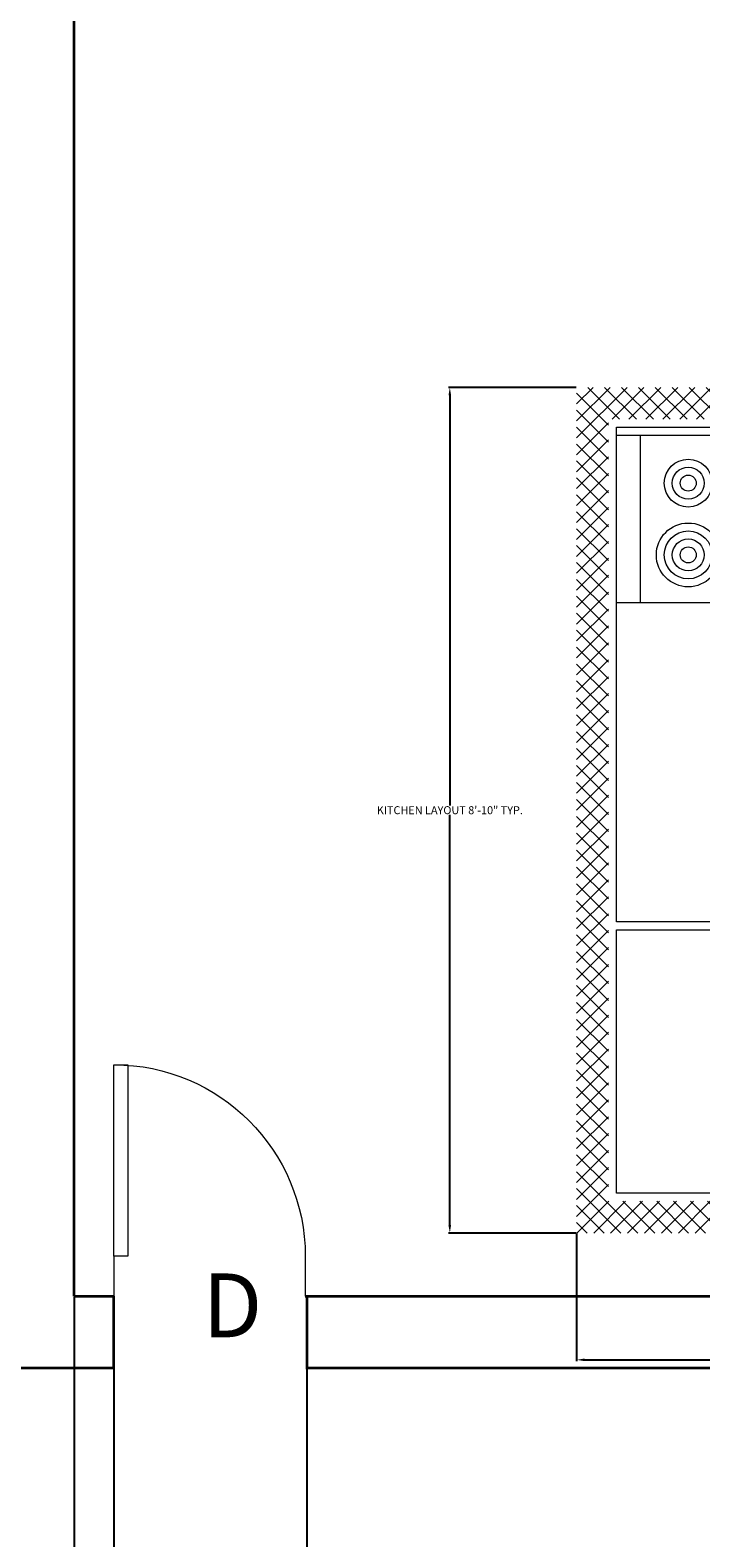
# Model space of a CAD drawing. Units: inches. Extents: x 371 to 1095, y -45 to 1219.
# Tile 11 of 18: x 856 to 940, y 421 to 610. Entities that reach past the tile are written whole.
import ezdxf

# ---------------------------------------------------------------- set-up
doc = ezdxf.new("R2010")
doc.units = ezdxf.units.IN
doc.header["$MEASUREMENT"] = 0
for name, color, linetype, lineweight in [('A-ANNO-DIMS', 2, 'Continuous', 18), ('A-ANNO-TEXT', 7, 'Continuous', 18), ('A-DOOR', 3, 'Continuous', 18), ('A-FLOR-FIXT', 9, 'Continuous', 18), ('A-WALL', 40, 'Continuous', 35)]:
    doc.layers.add(name, color=color, linetype=linetype, lineweight=lineweight)
doc.styles.get("Standard").update_dxf_attribs({"font": 'arial.ttf'})
doc.dimstyles.get("Standard").update_dxf_attribs({"dimtxt": 1, "dimasz": 1, "dimexe": 0.18, "dimexo": 0.0625, "dimgap": 0.09, "dimtad": 0, "dimtih": 1, "dimtoh": 1, "dimdec": 0, "dimzin": 0, "dimdsep": 46, "dimlunit": 3, "dimtxsty": 'Standard', "dimcen": 0.09, "dimadec": 0, "dimazin": 0, "dimtfac": 1, "dimtdec": 0, "dimtofl": 0, "dimtmove": 0, "dimatfit": 3, "dimfxl": 1, "dimtolj": 1, "dimtzin": 0, "dimarcsym": 0})

# ---------------------------------------------------------------- blocks, each defined once
blk = doc.blocks.new('*U12')
for p, q in [((0, 0), (0, 5)), ((24, 0), (24, 5))]:
    blk.add_line(p, q)
blk.add_lwpolyline([(0, 0), (0, -24), (1.75, -24), (1.75, 0)], close=True)
blk.add_arc((0, 0), 24, 270, 0)
blk = doc.blocks.new('Kitchen Layout - 7 x 8 ft')
for p, q in [((-5, 81.32), (2.68, 89)), ((-5, 83.44), (0.56, 89)), ((-5, 85.56), (-1.56, 89)), ((-5, 87.68), (-3.68, 89)), ((-1, 84.97), (-5, 88.97)), ((1.09, 85), (-2.91, 89)), ((3.21, 85), (-0.79, 89)), ((0.81, 85), (4.81, 89)), ((5.34, 85), (1.34, 89)), ((2.93, 85), (6.93, 89)), ((7.46, 85), (3.46, 89)), ((5.05, 85), (9.05, 89)), ((9.58, 85), (5.58, 89)), ((7.17, 85), (11.17, 89)), ((11.7, 85), (7.7, 89)), ((9.29, 85), (13.29, 89)), ((13.82, 85), (9.82, 89)), ((11.41, 85), (15.41, 89)), ((15.94, 85), (11.94, 89)), ((13.53, 85), (17.53, 89)), ((18.06, 85), (14.06, 89)), ((15.65, 85), (19.65, 89)), ((20.18, 85), (16.18, 89)), ((17.78, 85), (21.78, 89)), ((22.31, 85), (18.31, 89)), ((19.9, 85), (23.9, 89)), ((24.43, 85), (20.43, 89)), ((22.02, 85), (26.02, 89)), ((26.55, 85), (22.55, 89)), ((24.14, 85), (28.14, 89)), ((28.67, 85), (24.67, 89)), ((26.26, 85), (30.26, 89)), ((30.79, 85), (26.79, 89)), ((28.38, 85), (32.38, 89)), ((32.91, 85), (28.91, 89)), ((30.5, 85), (34.5, 89)), ((35.03, 85), (31.03, 89)), ((32.63, 85), (36.63, 89)), ((37.16, 85), (33.16, 89)), ((34.75, 85), (38.75, 89)), ((39.28, 85), (35.28, 89)), ((36.87, 85), (40.87, 89)), ((41.4, 85), (37.4, 89)), ((38.99, 85), (42.99, 89)), ((43.52, 85), (39.52, 89)), ((41.11, 85), (45.11, 89)), ((45.64, 85), (41.64, 89)), ((43.23, 85), (47.23, 89)), ((47.76, 85), (43.76, 89)), ((45.35, 85), (49.35, 89)), ((49.88, 85), (45.88, 89)), ((47.47, 85), (51.47, 89)), ((52, 85), (48, 89)), ((49.6, 85), (53.6, 89)), ((54.13, 85), (50.13, 89)), ((51.72, 85), (55.72, 89)), ((56.25, 85), (52.25, 89)), ((53.84, 85), (57.84, 89)), ((58.37, 85), (54.37, 89)), ((55.96, 85), (59.96, 89)), ((60.49, 85), (56.49, 89)), ((58.08, 85), (62.08, 89)), ((62.61, 85), (58.61, 89)), ((60.2, 85), (64.2, 89)), ((64.73, 85), (60.73, 89)), ((62.32, 85), (66.32, 89)), ((66.85, 85), (62.85, 89)), ((64.45, 85), (68.45, 89)), ((68.97, 85), (64.97, 89)), ((66.57, 85), (70.57, 89)), ((71.1, 85), (67.1, 89)), ((68.69, 85), (72.69, 89)), ((73.22, 85), (69.22, 89)), ((70.81, 85), (74.81, 89)), ((75.34, 85), (71.34, 89)), ((72.93, 85), (76.93, 89)), ((77.46, 85), (73.46, 89)), ((75.05, 85), (79.05, 89)), ((79.58, 85), (75.58, 89)), ((77.17, 85), (81.17, 89)), ((81.7, 85), (77.7, 89)), ((79.29, 85), (83.29, 89)), ((83.82, 85), (79.82, 89)), ((81.42, 85), (85.42, 89)), ((85.95, 85), (81.95, 89)), ((83.54, 85), (87.54, 89)), ((88.07, 85), (84.07, 89)), ((85.66, 85), (89.66, 89)), ((90.19, 85), (86.19, 89)), ((87.78, 85), (91.78, 89)), ((92.31, 85), (88.31, 89)), ((89.9, 85), (93.9, 89)), ((94.43, 85), (90.43, 89)), ((92.02, 85), (96.02, 89)), ((96.55, 85), (92.55, 89)), ((94.14, 85), (98.14, 89)), ((101, 82.67), (94.67, 89)), ((96.27, 85), (100.27, 89)), ((101, 84.79), (96.79, 89)), ((101, 86.92), (98.92, 89)), ((97, 83.61), (101, 87.61)), ((-1, 82.85), (-5, 86.85)), ((97, 81.49), (101, 85.49)), ((-1, 80.73), (-5, 84.73)), ((-5, 79.19), (-1, 83.19)), ((34, 84), (96, 84)), ((34, 60), (34, 84)), ((96, 84), (96, 60)), ((101, 80.55), (97, 84.55)), ((97, 79.37), (101, 83.37)), ((-1, 78.61), (-5, 82.61)), ((101, 78.43), (97, 82.43)), ((-5, 77.07), (-1, 81.07)), ((-1, 76.49), (-5, 80.49)), ((74, 81), (95, 81)), ((97, 77.25), (101, 81.25)), ((101, 76.31), (97, 80.31)), ((-5, 74.95), (-1, 78.95)), ((-1, 74.36), (-5, 78.36)), ((97, 75.13), (101, 79.13)), ((101, 74.19), (97, 78.19)), ((-5, 72.83), (-1, 76.83)), ((-1, 72.24), (-5, 76.24)), ((97, 73.01), (101, 77.01)), ((101, 72.07), (97, 76.07)), ((-5, 70.71), (-1, 74.71)), ((-1, 70.12), (-5, 74.12)), ((97, 70.89), (101, 74.89)), ((101, 69.95), (97, 73.95)), ((-5, 68.59), (-1, 72.59)), ((-1, 68), (-5, 72)), ((97, 68.76), (101, 72.76)), ((101, 67.82), (97, 71.82)), ((-5, 66.47), (-1, 70.47)), ((97, 66.64), (101, 70.64)), ((-1, 65.88), (-5, 69.88)), ((-5, 64.35), (-1, 68.35)), ((101, 65.7), (97, 69.7)), ((97, 64.52), (101, 68.52)), ((-1, 63.76), (-5, 67.76)), ((-5, 62.22), (-1, 66.22)), ((101, 63.58), (97, 67.58)), ((97, 62.4), (101, 66.4)), ((-1, 61.64), (-5, 65.64)), ((101, 61.46), (97, 65.46)), ((97, 60.28), (101, 64.28)), ((-5, 60.1), (-1, 64.1)), ((-1, 59.52), (-5, 63.52)), ((100.34, 60), (97, 63.34)), ((-5, 57.98), (-1, 61.98)), ((-1, 57.39), (-5, 61.39)), ((98.22, 60), (97, 61.22)), ((98.84, 60), (101, 62.16)), ((-1.73, 56), (-5, 59.27)), ((-4.86, 56), (-1, 59.86)), ((10.4, 24), (45.9, 59.5)), ((18.88, 24), (54.38, 59.5)), ((27.37, 24), (62.87, 59.5)), ((33.03, 55.11), (37.41, 59.5)), ((96, 60), (34, 60)), ((35.85, 24), (71.35, 59.5)), ((76.2, 24), (40.7, 59.5)), ((84.68, 24), (49.18, 59.5)), ((93.17, 24), (57.67, 59.5)), ((61.31, 24), (96, 58.69)), ((96, 29.65), (66.15, 59.5)), ((80, 60), (80, 59)), ((82, 59), (82, 60)), ((87, 59), (87, 60)), ((89, 60), (89, 59)), ((100.96, 60), (101, 60.04)), ((-3.85, 56), (-5, 57.15)), ((-2.74, 56), (-1, 57.74)), ((0, 57), (33, 57)), ((67.71, 24), (33.68, 58.04)), ((44.34, 24), (77.84, 57.5)), ((52.82, 24), (86.32, 57.5)), ((96, 38.14), (76.64, 57.5)), ((96, 46.63), (85.13, 57.5)), ((96, 55.11), (93.57, 57.54)), ((0, 30.57), (24.43, 55)), ((0, 39.06), (15.94, 55)), ((0, 47.54), (7.46, 55)), ((1.91, 24), (32.91, 55)), ((33.77, 24), (2.77, 55)), ((42.26, 24), (11.26, 55)), ((50.74, 24), (19.74, 55)), ((59.23, 24), (28.23, 55)), ((31, 55), (31, 56)), ((32, 55), (31, 55)), ((32, 56), (32, 55)), ((25.29, 24), (0, 49.29)), ((69.79, 24), (96, 50.21)), ((78.28, 24), (96, 41.72)), ((16.8, 24), (0, 40.8)), ((8.32, 24), (0, 32.32)), ((86.76, 24), (96, 33.24)), ((95.25, 24), (96, 24.75)), ((-5, 21.92), (-2.92, 24)), ((-5, 19.8), (-1, 23.8)), ((-1, 19.21), (-5, 23.21)), ((-1, 21.33), (-3.67, 24)), ((-1, 23.45), (-1.55, 24)), ((0, 24), (96, 24)), ((0, 0), (0, 24)), ((96, 24), (96, 0)), ((97, 22.1), (98.9, 24)), ((97, 19.97), (101, 23.97)), ((101, 19.03), (97, 23.03)), ((101, 21.16), (98.16, 24)), ((101, 23.28), (100.28, 24)), ((-5, 17.68), (-1, 21.68)), ((-1, 17.09), (-5, 21.09)), ((97, 17.85), (101, 21.85)), ((101, 16.91), (97, 20.91)), ((-5, 15.55), (-1, 19.55)), ((-1, 14.97), (-5, 18.97)), ((97, 15.73), (101, 19.73)), ((-5, 13.43), (-1, 17.43)), ((47.25, 6.5), (47.25, 18.5)), ((48.75, 18.5), (48.75, 6.5)), ((101, 14.79), (97, 18.79)), ((97, 13.61), (101, 17.61)), ((-1, 12.85), (-5, 16.85)), ((-5, 11.31), (-1, 15.31)), ((101, 12.67), (97, 16.67)), ((97, 11.49), (101, 15.49)), ((-1, 10.73), (-5, 14.73)), ((101, 10.55), (97, 14.55)), ((97, 9.37), (101, 13.37)), ((-5, 9.19), (-1, 13.19)), ((-1, 8.6), (-5, 12.6)), ((101, 8.43), (97, 12.43)), ((-5, 7.07), (-1, 11.07)), ((-1, 6.48), (-5, 10.48)), ((97, 7.25), (101, 11.25)), ((101, 6.31), (97, 10.31)), ((-5, 4.95), (-1, 8.95)), ((-1, 4.36), (-5, 8.36)), ((97, 5.12), (101, 9.12)), ((101, 4.18), (97, 8.18)), ((-5, 2.83), (-1, 6.83)), ((-1, 2.24), (-5, 6.24)), ((97, 3), (101, 7)), ((101, 2.06), (97, 6.06)), ((-5, 0.71), (-1, 4.71)), ((-1, 0.12), (-5, 4.12)), ((64, 4), (32, 4)), ((97, 0.88), (101, 4.88)), ((101, -0.06), (97, 3.94)), ((-5, -1.42), (-1, 2.58)), ((2, -5), (-5, 2)), ((93.24, -5), (101, 2.76)), ((-5, -3.54), (-1, 0.46)), ((96, 0), (0, 0)), ((95.36, -5), (101, 0.64)), ((101, -2.18), (97, 1.82)), ((-0.12, -5), (-5, -0.12)), ((-4.34, -5), (-0.34, -1)), ((-2.22, -5), (1.78, -1)), ((-0.1, -5), (3.9, -1)), ((4.12, -5), (0.12, -1)), ((2.02, -5), (6.02, -1)), ((6.24, -5), (2.24, -1)), ((4.14, -5), (8.14, -1)), ((8.36, -5), (4.36, -1)), ((6.27, -5), (10.27, -1)), ((10.48, -5), (6.48, -1)), ((8.39, -5), (12.39, -1)), ((12.6, -5), (8.6, -1)), ((10.51, -5), (14.51, -1)), ((14.73, -5), (10.73, -1)), ((12.63, -5), (16.63, -1)), ((16.85, -5), (12.85, -1)), ((14.75, -5), (18.75, -1)), ((18.97, -5), (14.97, -1)), ((16.87, -5), (20.87, -1)), ((21.09, -5), (17.09, -1)), ((18.99, -5), (22.99, -1)), ((23.21, -5), (19.21, -1)), ((21.11, -5), (25.11, -1)), ((25.33, -5), (21.33, -1)), ((23.24, -5), (27.24, -1)), ((27.45, -5), (23.45, -1)), ((25.36, -5), (29.36, -1)), ((29.57, -5), (25.57, -1)), ((30, -3.3), (27.7, -1)), ((30, -1.18), (29.82, -1)), ((66, -2.54), (67.54, -1)), ((66, -4.66), (69.66, -1)), ((69.88, -5), (66, -1.12)), ((67.78, -5), (71.78, -1)), ((72, -5), (68, -1)), ((69.9, -5), (73.9, -1)), ((74.12, -5), (70.12, -1)), ((72.03, -5), (76.03, -1)), ((76.24, -5), (72.24, -1)), ((74.15, -5), (78.15, -1)), ((78.36, -5), (74.36, -1)), ((76.27, -5), (80.27, -1)), ((80.49, -5), (76.49, -1)), ((78.39, -5), (82.39, -1)), ((82.61, -5), (78.61, -1)), ((80.51, -5), (84.51, -1)), ((84.73, -5), (80.73, -1)), ((82.63, -5), (86.63, -1)), ((86.85, -5), (82.85, -1)), ((84.75, -5), (88.75, -1)), ((88.97, -5), (84.97, -1)), ((86.88, -5), (90.88, -1)), ((91.09, -5), (87.09, -1)), ((89, -5), (93, -1)), ((93.21, -5), (89.21, -1)), ((91.12, -5), (95.12, -1)), ((95.34, -5), (91.34, -1)), ((97.46, -5), (93.46, -1)), ((99.58, -5), (95.58, -1)), ((101, -4.3), (97, -0.3)), ((97.48, -5), (101, -1.48)), ((-2.25, -5), (-5, -2.25)), ((27.48, -5), (30, -2.48)), ((67.76, -5), (66, -3.24)), ((99.6, -5), (101, -3.6)), ((-4.37, -5), (-5, -4.37)), ((29.6, -5), (30, -4.6))]:
    blk.add_line(p, q)
for points in [[(0, 56), (0, 84), (33, 84), (33, 56)], [(74, 60), (74, 84), (95, 84), (95, 60)], [(76, 58), (76, 59), (93, 59), (93, 58)]]:
    blk.add_lwpolyline(points, close=True)
for points in [[(33.5, 21), (62.5, 21)], [(32, 1.5), (32, 19.5)], [(34.5, 19.5), (46.25, 19.5)], [(49.75, 19.5), (61.5, 19.5)], [(64, 19.5), (64, 1.5)], [(33.5, 6.5), (33.5, 18.5)], [(62.5, 18.5), (62.5, 6.5)], [(46.25, 5.5), (34.5, 5.5)], [(61.5, 5.5), (49.75, 5.5)], [(62.5, 0), (33.5, 0)]]:
    blk.add_lwpolyline(points)
for centre, radius in [((80, 75), 4), ((80, 75), 3), ((89, 75), 3), ((80, 75), 2), ((80, 75), 1), ((89, 75), 2), ((89, 75), 1), ((89, 66), 4), ((80, 66), 3), ((89, 66), 3), ((80, 66), 2), ((80, 66), 1), ((89, 66), 2), ((89, 66), 1), ((40.5, 12.5), 1), ((55.5, 12.5), 1), ((40.5, 12.5), 0.5), ((55.5, 12.5), 0.5)]:
    blk.add_circle(centre, radius)
for centre, radius, start, end in [((33.5, 19.5), 1.5, 90, 180), ((62.5, 19.5), 1.5, 0, 90), ((34.5, 18.5), 1, 90, 180), ((46.25, 18.5), 1, 0, 90), ((49.75, 18.5), 1, 90, 180), ((61.5, 18.5), 1, 0, 90), ((34.5, 6.5), 1, 180, 270), ((46.25, 6.5), 1, 270, 0), ((49.75, 6.5), 1, 180, 270), ((61.5, 6.5), 1, 270, 0), ((33.5, 1.5), 1.5, 180, 270), ((62.5, 1.5), 1.5, 270, 0)]:
    blk.add_arc(centre, radius, start, end)
blk = doc.blocks.new('*D36')
at = {"layer": 'A-ANNO-DIMS', "color": 0, "lineweight": -2, "transparency": 16777216}
for p, q in [((924.77, 564.94), (908.76, 564.94)), ((908.94, 563.94), (908.94, 512.55)), ((908.94, 459.94), (908.94, 511.34)), ((924.77, 458.94), (908.76, 458.94))]:
    blk.add_line(p, q, dxfattribs=at)
at = {"layer": 'A-ANNO-DIMS', "color": 0, "transparency": 16777216}
for points in [[(908.77, 563.94), (909.1, 563.94), (908.94, 564.94)], [(908.77, 459.94), (909.1, 459.94), (908.94, 458.94)]]:
    blk.add_solid(points, dxfattribs=at)
at = {"layer": 'Defpoints', "color": 0, "transparency": 16777216}
for p in [(908.94, 564.94), (924.84, 564.94), (924.84, 458.94)]:
    blk.add_point(p, dxfattribs=at)
at = {"layer": 'A-ANNO-DIMS', "color": 0, "transparency": 16777216, "insert": (908.94, 511.94), "char_height": 1, "attachment_point": 5}
blk.add_mtext('\\A1;KITCHEN LAYOUT 8\'-10" TYP.', dxfattribs=at)
blk = doc.blocks.new('*D37')
at = {"layer": 'A-ANNO-DIMS', "color": 0, "lineweight": -2, "transparency": 16777216}
for p, q in [((924.84, 458.88), (924.84, 442.86)), ((1018.84, 458.88), (1018.84, 442.86)), ((925.84, 443.04), (968.31, 443.04)), ((1017.84, 443.04), (975.36, 443.04))]:
    blk.add_line(p, q, dxfattribs=at)
at = {"layer": 'A-ANNO-DIMS', "color": 0, "transparency": 16777216}
for points in [[(925.84, 443.21), (925.84, 442.88), (924.84, 443.04)], [(1017.84, 443.21), (1017.84, 442.88), (1018.84, 443.04)]]:
    blk.add_solid(points, dxfattribs=at)
at = {"layer": 'Defpoints', "color": 0, "transparency": 16777216}
for p in [(924.84, 458.94), (1018.84, 458.94), (924.84, 443.04)]:
    blk.add_point(p, dxfattribs=at)
at = {"layer": 'A-ANNO-DIMS', "color": 0, "transparency": 16777216, "insert": (971.84, 443.04), "char_height": 1, "attachment_point": 5}
blk.add_mtext('\\A1;7\'-10" TYP.', dxfattribs=at)
blk = doc.blocks.new('*D60')
at = {"layer": 'A-ANNO-DIMS', "color": 0, "lineweight": -2, "transparency": 16777216}
for p, q in [((866.81, 441.96), (866.81, -43.83)), ((891.01, 441.96), (891.01, -43.83)), ((867.81, -43.65), (877.48, -43.65)), ((890.01, -43.65), (880.33, -43.65))]:
    blk.add_line(p, q, dxfattribs=at)
at = {"layer": 'A-ANNO-DIMS', "color": 0, "transparency": 16777216}
for points in [[(867.81, -43.48), (867.81, -43.82), (866.81, -43.65)], [(890.01, -43.48), (890.01, -43.82), (891.01, -43.65)]]:
    blk.add_solid(points, dxfattribs=at)
at = {"layer": 'Defpoints', "color": 0, "transparency": 16777216}
for p in [(866.81, 442.03), (891.01, 442.03), (891.01, -43.65)]:
    blk.add_point(p, dxfattribs=at)
at = {"layer": 'A-ANNO-DIMS', "color": 0, "transparency": 16777216, "insert": (878.91, -43.65), "char_height": 1, "attachment_point": 5}
blk.add_mtext('\\A1;2\'-0"', dxfattribs=at)
blk = doc.blocks.new('*D61')
at = {"layer": 'A-ANNO-DIMS', "color": 0, "lineweight": -2, "transparency": 16777216}
for p, q in [((861.81, 450.96), (861.81, -43.83)), ((866.81, 450.96), (866.81, -43.83)), ((860.81, -43.65), (859.81, -43.65)), ((867.81, -43.65), (868.81, -43.65))]:
    blk.add_line(p, q, dxfattribs=at)
at = {"layer": 'A-ANNO-DIMS', "color": 0, "transparency": 16777216}
for points in [[(860.81, -43.48), (860.81, -43.82), (861.81, -43.65)], [(867.81, -43.48), (867.81, -43.82), (866.81, -43.65)]]:
    blk.add_solid(points, dxfattribs=at)
at = {"layer": 'Defpoints', "color": 0, "transparency": 16777216}
for p in [(861.81, 451.03), (866.81, 451.03), (866.81, -43.65)]:
    blk.add_point(p, dxfattribs=at)
at = {"layer": 'A-ANNO-DIMS', "color": 0, "transparency": 16777216, "insert": (864.31, -43.65), "char_height": 1, "attachment_point": 5}
blk.add_mtext('\\A1;0\'-5"', dxfattribs=at)

msp = doc.modelspace()

# ---------------------------------------------------------------- linework, layer by layer
at = {"layer": 'A-WALL'}
for p, q in [((861.81, 451.03), (861.81, 796.03)), ((861.81, 451.03), (866.81, 451.03)), ((866.81, 442.03), (866.81, 451.03)), ((890.81, 451.03), (1023.81, 451.03)), ((891.01, 450.88), (891.01, 441.88)), ((852.81, 442.03), (866.81, 442.03)), ((891.01, 442.03), (1023.81, 442.03))]:
    msp.add_line(p, q, dxfattribs=at)

# ---------------------------------------------------------------- block references
at = {"layer": 'A-DOOR', "xscale": -1, "rotation": 180}
msp.add_blockref('*U12', (866.81, 456.03), dxfattribs=at)
at = {"layer": 'A-FLOR-FIXT', "rotation": 89.99999999999999}
msp.add_blockref('Kitchen Layout - 7 x 8 ft', (1013.84, 463.94), dxfattribs=at)

# ---------------------------------------------------------------- texts
at = {"layer": 'A-ANNO-TEXT', "insert": (877.91, 453.87), "char_height": 8, "attachment_point": 1}
msp.add_mtext_dynamic_manual_height_columns('D', width=17.4938, gutter_width=1, heights=[0], dxfattribs=at)

# ---------------------------------------------------------------- dimensions: what is measured, and where the dimension line sits
at = {"layer": 'A-ANNO-DIMS'}
for base, p1, p2, angle, text, picture, middle in [((908.94, 564.94), (924.84, 458.94), (924.84, 564.94), 90, 'KITCHEN LAYOUT <> TYP.', '*D36', (908.94, 511.94)), ((924.84, 443.04), (1018.84, 458.94), (924.84, 458.94), 180, '<> TYP.', '*D37', (971.84, 443.04))]:
    dim = msp.add_linear_dim(base=base, p1=p1, p2=p2, angle=angle, text=text, dimstyle='Standard', override={"dimdec": 1, "dimlfac": 1, "dimrnd": 0, "dimzin": 1, "dimdsep": 46, "dimlunit": 4, "dimfrac": 2}, dxfattribs=at)
    dim.commit()
    dim.dimension.update_dxf_attribs({"geometry": picture, "text_midpoint": middle})
for base, p1, p2, picture, middle in [((866.81, -43.65), (861.81, 451.03), (866.81, 451.03), '*D61', (864.31, -43.65)), ((891.01, -43.65), (866.81, 442.03), (891.01, 442.03), '*D60', (878.91, -43.65))]:
    dim = msp.add_linear_dim(base=base, p1=p1, p2=p2, dimstyle='Standard', override={"dimdec": 1, "dimlfac": 1, "dimrnd": 0, "dimzin": 1, "dimdsep": 46, "dimlunit": 4, "dimfrac": 2}, dxfattribs=at)
    dim.commit()
    dim.dimension.update_dxf_attribs({"geometry": picture, "text_midpoint": middle})

doc.saveas('drawing.dxf')
